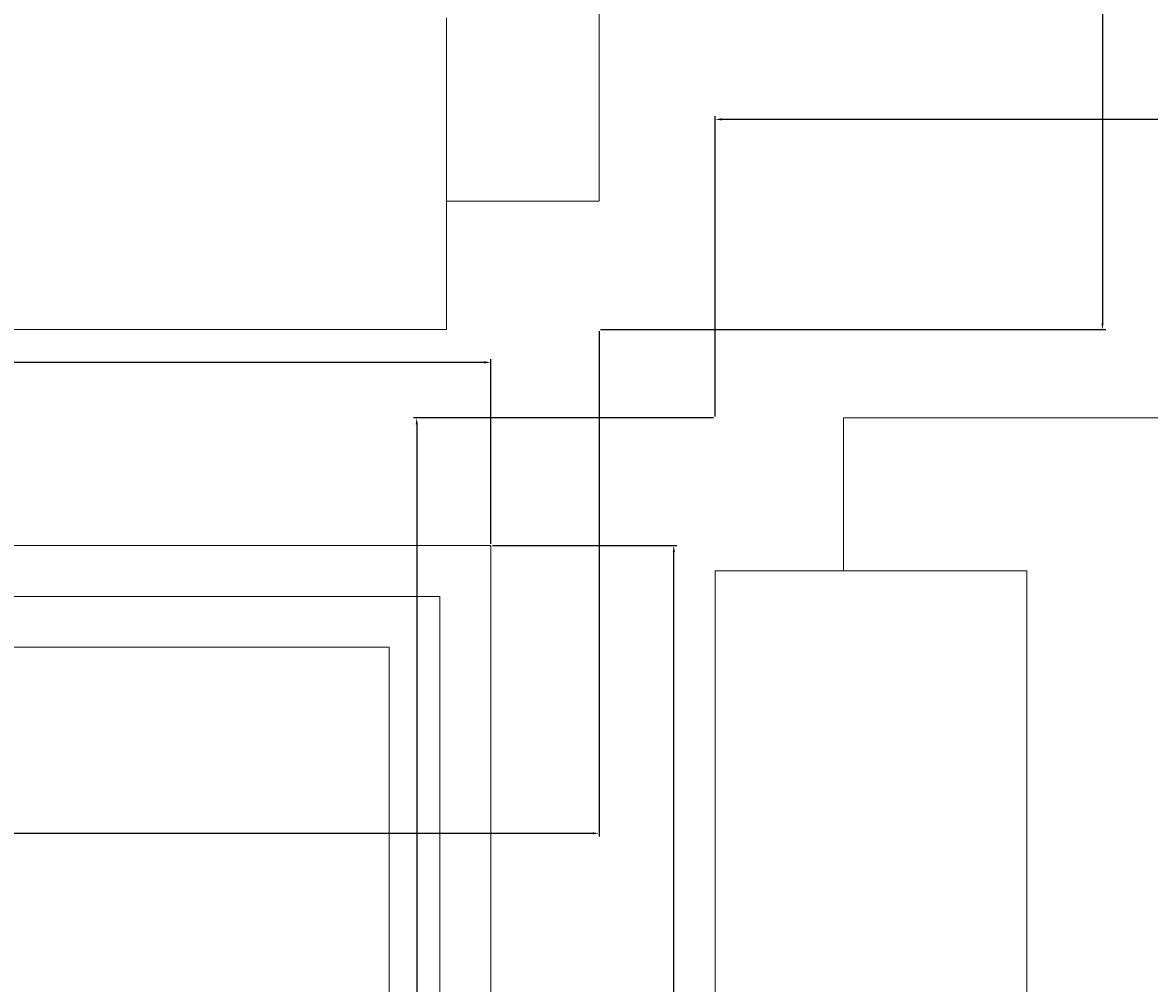
# Model space of a CAD drawing. Units: millimetres. Extents: x -857 to 54106, y -13666 to 13947.
# Tile 7 of 41: x 7861 to 8305, y 6612 to 6990. Entities that reach past the tile are written whole.
import ezdxf

# ---------------------------------------------------------------- set-up
doc = ezdxf.new("R2010")
doc.units = ezdxf.units.MM
for name, color, linetype, lineweight in [('A-ANNO-DIMS', 2, 'Continuous', 18), ('A-FURN', 21, 'Continuous', 18), ('A-FURNITURE', 25, 'Continuous', 9)]:
    doc.layers.add(name, color=color, linetype=linetype, lineweight=lineweight)
doc.styles.get("Standard").update_dxf_attribs({"font": 'arial.ttf'})
doc.dimstyles.new('ISO-25', dxfattribs={"dimtxt": 2.5, "dimasz": 2.5, "dimexe": 1.25, "dimexo": 0.625, "dimtad": 1, "dimtxsty": 'Standard', "dimcen": 2.5, "dimadec": 0, "dimazin": 0, "dimtfac": 1, "dimtmove": 0, "dimatfit": 3, "dimfxl": 1, "dimarcsym": 0})

# ---------------------------------------------------------------- blocks, each defined once
blk = doc.blocks.new('A$C0E8E2537')
at = {"layer": 'A-FURNITURE'}
for p, q in [((33, -5.045), (33, -26.997)), ((33, -26.997), (26.874, -26.997)), ((30.478, -26.997), (30.478, -30)), ((30.478, -30), (-30.478, -30))]:
    blk.add_line(p, q, dxfattribs=at)
blk = doc.blocks.new('A$C21FE29A1')
at = {"layer": 'A-FURNITURE'}
for points in [[(0, 0), (24, 0), (24, 24), (0, 24)], [(1, 1), (23, 1), (23, 23), (1, 23)], [(2, 2), (22, 2), (22, 22), (2, 22)]]:
    blk.add_lwpolyline(points, close=True, dxfattribs=at)
blk = doc.blocks.new('A$C47E27A62')
at = {"layer": 'A-FURNITURE'}
for p, q in [((19.563, -5.045), (19.563, -26.997)), ((13.437, -6.486), (13.437, -26.997)), ((19.563, -26.997), (13.437, -26.997)), ((17.041, -26.997), (17.041, -30)), ((17.041, -30), (-17.041, -30))]:
    blk.add_line(p, q, dxfattribs=at)
blk = doc.blocks.new('*D53')
at = {"layer": 'A-ANNO-DIMS', "color": 0, "lineweight": -2, "transparency": 16777216}
for p, q in [((8089.06, 8191.6), (8288.04, 8191.6)), ((8286.79, 8189.1), (8286.79, 6871.69)), ((8089.06, 6869.19), (8288.04, 6869.19))]:
    blk.add_line(p, q, dxfattribs=at)
at = {"layer": 'A-ANNO-DIMS', "color": 0, "transparency": 16777216}
for points in [[(8286.38, 8189.1), (8287.21, 8189.1), (8286.79, 8191.6)], [(8286.38, 6871.69), (8287.21, 6871.69), (8286.79, 6869.19)]]:
    blk.add_solid(points, dxfattribs=at)
at = {"layer": 'Defpoints', "color": 0, "transparency": 16777216}
for p in [(8088.43, 8191.6), (8088.43, 6869.19), (8286.79, 6869.19)]:
    blk.add_point(p, dxfattribs=at)
at = {"layer": 'A-ANNO-DIMS', "color": 0, "transparency": 16777216, "insert": (8284.87, 7530.39), "char_height": 2.5, "attachment_point": 5, "rotation": 90}
blk.add_mtext('SOFA 1322', dxfattribs=at)
blk = doc.blocks.new('*D54')
at = {"layer": 'A-ANNO-DIMS', "color": 0, "lineweight": -2, "transparency": 16777216}
for p, q in [((7487.34, 6868.56), (7487.34, 6669.58)), ((8088.43, 6868.56), (8088.43, 6669.58)), ((8085.93, 6670.83), (7489.84, 6670.83))]:
    blk.add_line(p, q, dxfattribs=at)
at = {"layer": 'A-ANNO-DIMS', "color": 0, "transparency": 16777216}
for points in [[(7489.84, 6671.24), (7489.84, 6670.41), (7487.34, 6670.83)], [(8085.93, 6671.24), (8085.93, 6670.41), (8088.43, 6670.83)]]:
    blk.add_solid(points, dxfattribs=at)
at = {"layer": 'Defpoints', "color": 0, "transparency": 16777216}
for p in [(7487.34, 6869.19), (8088.43, 6869.19), (7487.34, 6670.83)]:
    blk.add_point(p, dxfattribs=at)
at = {"layer": 'A-ANNO-DIMS', "color": 0, "transparency": 16777216, "insert": (7787.89, 6672.73), "char_height": 2.5, "attachment_point": 5}
blk.add_mtext('601', dxfattribs=at)
blk = doc.blocks.new('*D57')
at = {"layer": 'A-ANNO-DIMS', "color": 0, "lineweight": -2, "transparency": 16777216}
for p, q in [((7564.88, 6784.8), (7564.88, 6857.56)), ((8043.26, 6856.31), (7567.38, 6856.31)), ((8045.76, 6784.8), (8045.76, 6857.56))]:
    blk.add_line(p, q, dxfattribs=at)
at = {"layer": 'A-ANNO-DIMS', "color": 0, "transparency": 16777216}
for points in [[(7567.38, 6856.72), (7567.38, 6855.89), (7564.88, 6856.31)], [(8043.26, 6856.72), (8043.26, 6855.89), (8045.76, 6856.31)]]:
    blk.add_solid(points, dxfattribs=at)
at = {"layer": 'Defpoints', "color": 0, "transparency": 16777216}
for p in [(7564.88, 6856.31), (7564.88, 6784.17), (8045.76, 6784.17)]:
    blk.add_point(p, dxfattribs=at)
at = {"layer": 'A-ANNO-DIMS', "color": 0, "transparency": 16777216, "insert": (7805.32, 6858.22), "char_height": 2.5, "attachment_point": 5}
blk.add_mtext('SIDE TABLE 481', dxfattribs=at)
blk = doc.blocks.new('*D58')
at = {"layer": 'A-ANNO-DIMS', "color": 0, "lineweight": -2, "transparency": 16777216}
for p, q in [((8046.39, 6784.17), (8119.14, 6784.17)), ((8117.89, 6305.8), (8117.89, 6781.67)), ((8046.39, 6303.3), (8119.14, 6303.3))]:
    blk.add_line(p, q, dxfattribs=at)
at = {"layer": 'A-ANNO-DIMS', "color": 0, "transparency": 16777216}
for points in [[(8117.48, 6781.67), (8118.31, 6781.67), (8117.89, 6784.17)], [(8117.48, 6305.8), (8118.31, 6305.8), (8117.89, 6303.3)]]:
    blk.add_solid(points, dxfattribs=at)
at = {"layer": 'Defpoints', "color": 0, "transparency": 16777216}
for p in [(8045.76, 6784.17), (8117.89, 6784.17), (8045.76, 6303.3)]:
    blk.add_point(p, dxfattribs=at)
at = {"layer": 'A-ANNO-DIMS', "color": 0, "transparency": 16777216, "insert": (8115.99, 6543.74), "char_height": 2.5, "attachment_point": 5, "rotation": 90}
blk.add_mtext('481', dxfattribs=at)
blk = doc.blocks.new('*D59')
at = {"layer": 'A-ANNO-DIMS', "color": 0, "lineweight": -2, "transparency": 16777216}
for p, q in [((8134.19, 6835.03), (8134.19, 6953.24)), ((8918.14, 6835.03), (8918.14, 6953.24)), ((8915.64, 6951.99), (8136.69, 6951.99))]:
    blk.add_line(p, q, dxfattribs=at)
at = {"layer": 'A-ANNO-DIMS', "color": 0, "transparency": 16777216}
for points in [[(8136.69, 6952.41), (8136.69, 6951.58), (8134.19, 6951.99)], [(8915.64, 6952.41), (8915.64, 6951.58), (8918.14, 6951.99)]]:
    blk.add_solid(points, dxfattribs=at)
at = {"layer": 'Defpoints', "color": 0, "transparency": 16777216}
for p in [(8134.19, 6951.99), (8134.19, 6834.4), (8918.14, 6834.4)]:
    blk.add_point(p, dxfattribs=at)
at = {"layer": 'A-ANNO-DIMS', "color": 0, "transparency": 16777216, "insert": (8526.17, 6953.91), "char_height": 2.5, "attachment_point": 5}
blk.add_mtext('COFFEE TABLE 784', dxfattribs=at)
blk = doc.blocks.new('*D60')
at = {"layer": 'A-ANNO-DIMS', "color": 0, "lineweight": -2, "transparency": 16777216}
for p, q in [((8133.57, 6834.4), (8015.35, 6834.4)), ((8016.6, 6831.9), (8016.6, 6235.81)), ((8133.57, 6233.31), (8015.35, 6233.31))]:
    blk.add_line(p, q, dxfattribs=at)
at = {"layer": 'A-ANNO-DIMS', "color": 0, "transparency": 16777216}
for points in [[(8016.19, 6831.9), (8017.02, 6831.9), (8016.6, 6834.4)], [(8016.19, 6235.81), (8017.02, 6235.81), (8016.6, 6233.31)]]:
    blk.add_solid(points, dxfattribs=at)
at = {"layer": 'Defpoints', "color": 0, "transparency": 16777216}
for p in [(8134.19, 6834.4), (8016.6, 6233.31), (8134.19, 6233.31)]:
    blk.add_point(p, dxfattribs=at)
at = {"layer": 'A-ANNO-DIMS', "color": 0, "transparency": 16777216, "insert": (8014.7, 6533.85), "char_height": 2.5, "attachment_point": 5, "rotation": 90}
blk.add_mtext('601', dxfattribs=at)

msp = doc.modelspace()

# ---------------------------------------------------------------- block references
at = {"layer": 'A-FURN', "ltscale": 4}
for name, p, xscale, yscale, zscale, rotation in [('A$C0E8E2537', (7487.337, 7530.393), -20.03650789584554, 20.03650789584554, 20.03650789584554, 90), ('A$C47E27A62', (8526.165, 6233.305), 20.03650789584363, 20.03650789584363, 20.03650789584363, 180)]:
    msp.add_blockref(name, p, dxfattribs=dict(at, xscale=xscale, yscale=yscale, zscale=zscale, rotation=rotation))
at = {"layer": 'A-FURN', "xscale": 20.03650789584554, "yscale": 20.03650789584554, "zscale": 20.03650789584554, "rotation": 89.99999999999999}
msp.add_blockref('A$C21FE29A1', (8045.76, 6303.297), dxfattribs=at)

# ---------------------------------------------------------------- dimensions: what is measured, and where the dimension line sits
at = {"layer": 'A-ANNO-DIMS'}
for base, p1, p2, angle, text, picture, middle in [((8286.794, 6869.188), (8088.433, 8191.597), (8088.433, 6869.188), 270, 'SOFA <>', '*D53', (8284.875, 7530.393)), ((8134.194, 6951.992), (8918.137, 6834.4), (8134.194, 6834.4), 180, 'COFFEE TABLE <>', '*D59', (8526.165, 6953.91)), ((7564.885, 6856.306), (8045.761, 6784.175), (7564.885, 6784.175), 180, 'SIDE TABLE <>', '*D57', (7805.323, 6858.224))]:
    dim = msp.add_linear_dim(base=base, p1=p1, p2=p2, angle=angle, text=text, dimstyle='ISO-25', override={"dimdec": 0, "dimrnd": 0, "dimzin": 0, "dimlunit": 2}, dxfattribs=at)
    dim.commit()
    dim.dimension.update_dxf_attribs({"geometry": picture, "text_midpoint": middle})
for base, p1, p2, angle, picture, middle in [((7487.337, 6670.826), (8088.433, 6869.188), (7487.337, 6869.188), 180, '*D54', (7787.885, 6672.728)), ((8016.602, 6233.305), (8134.194, 6834.4), (8134.194, 6233.305), 270, '*D60', (8014.701, 6533.853)), ((8117.892, 6784.175), (8045.761, 6303.298), (8045.761, 6784.175), 90, '*D58', (8115.991, 6543.737))]:
    dim = msp.add_linear_dim(base=base, p1=p1, p2=p2, angle=angle, dimstyle='ISO-25', override={"dimdec": 0, "dimrnd": 0, "dimzin": 0, "dimlunit": 2}, dxfattribs=at)
    dim.commit()
    dim.dimension.update_dxf_attribs({"geometry": picture, "text_midpoint": middle})

doc.saveas('drawing.dxf')
